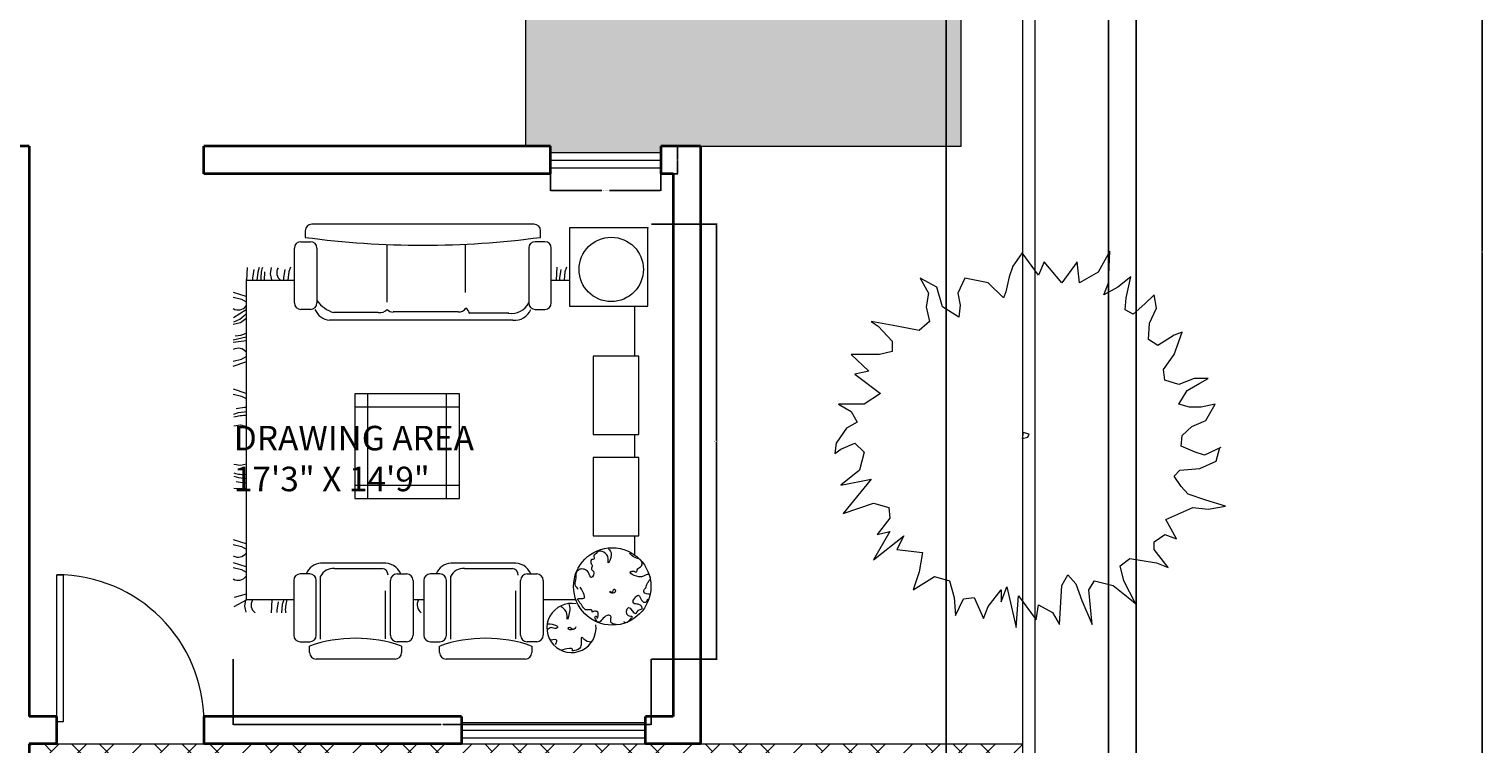
# Model space of a CAD drawing. Units: inches. Extents: x -4843 to -3402, y -164 to 3629.
# Tile 6 of 22: x -4303 to -3829, y 457 to 691. Entities that reach past the tile are written whole.
import ezdxf

# ---------------------------------------------------------------- set-up
doc = ezdxf.new("R2010")
doc.units = ezdxf.units.IN
for name, color, linetype, lineweight in [('A-ANNO-DIMS', 2, 'Continuous', 18), ('A-AREA-IDEN', 2, 'Continuous', 18), ('A-FLOR-DECK', 7, 'Continuous', 18), ('C-PROP', 7, 'Continuous', 25), ('C-PVMT', 7, 'Continuous', 18), ('doors', 2, 'Continuous', 18), ('furniture', 6, 'Continuous', 18), ('L-PLNT-EDGE', 7, 'Continuous', 18), ('PLANTS', 3, 'Continuous', 13), ('walls', 7, 'Continuous', 35), ('windows', 1, 'Continuous', 18)]:
    doc.layers.add(name, color=color, linetype=linetype, lineweight=lineweight)
doc.layers.add('A-FLOR-PATT', color=30, linetype='Continuous', lineweight=13, true_color=0xf26722)
doc.layers.add('C-PVMT-PATT', color=9, linetype='Continuous', lineweight=13, true_color=0xc7c8ca)
doc.styles.get("Standard").update_dxf_attribs({"font": 'arial.ttf'})
doc.dimstyles.get("Standard").update_dxf_attribs({"dimtxt": 0.18, "dimasz": 0.18, "dimexe": 0.18, "dimexo": 0.0625, "dimgap": 0.09, "dimtad": 0, "dimtih": 1, "dimtoh": 1, "dimdec": 4, "dimzin": 0, "dimdsep": 46, "dimtxsty": 'Standard', "dimcen": 0.09, "dimadec": 0, "dimazin": 0, "dimtfac": 1, "dimtdec": 4, "dimtofl": 0, "dimtmove": 0, "dimatfit": 3, "dimfxl": 1, "dimtolj": 1, "dimtzin": 0, "dimarcsym": 0})
pattern_1 = [(45, (-7766.296, -1992.247), (-4.490128, 4.490128), []), (135, (-7766.296, -1992.247), (-13.470384, 4.490128), [15.875, -9.525])]

# ---------------------------------------------------------------- blocks, each defined once
blk = doc.blocks.new('window')
at = {"layer": 'windows'}
for p, q in [((0, 7), (60, 7)), ((0, 4.5), (60, 4.5)), ((0, 2), (60, 2))]:
    blk.add_line(p, q, dxfattribs=at)
for points in [[(0, 9), (0, 0)], [(60, 0), (60, 9)]]:
    blk.add_lwpolyline(points, dxfattribs=at)
blk = doc.blocks.new('windw 3')
at = {"layer": 'windows'}
for p, q in [((0, 7), (36, 7)), ((0, 4.5), (36, 4.5)), ((0, 2), (36, 2))]:
    blk.add_line(p, q, dxfattribs=at)
for points in [[(0, 0), (0, 9)], [(36, 9), (36, 0)]]:
    blk.add_lwpolyline(points, dxfattribs=at)
blk = doc.blocks.new('*U7')
for p, q in [((0, 0), (0, -6)), ((40, 0), (40, -6))]:
    blk.add_line(p, q)
blk.add_lwpolyline([(0, 0), (0, 40), (1.75, 40), (1.75, 0)], close=True)
blk.add_arc((0, 0), 40, 0, 90)
blk = doc.blocks.new('A$C688935E4')
for p, q in [((552, 3277), (552, 3227)), ((2302, 3327), (602, 3327)), ((2352, 3227), (2352, 3277)), ((3173, 3300), (2573, 3300)), ((2573, 3300), (2573, 2700)), ((3173, 2700), (3173, 3300)), ((469, 2725), (469, 3144)), ((519, 3194), (592, 3194)), ((642, 3144), (642, 2725)), ((1175, 3172), (1175, 2731)), ((1775, 3172), (1775, 2805)), ((2261, 3144), (2261, 2725)), ((2384, 3194), (2311, 3194)), ((2434, 2725), (2434, 3144)), ((97, 2899), (469, 2899)), ((102, 454), (102, 2904)), ((108, 2997), (104, 2897)), ((158, 2980), (148, 2916)), ((148, 2916), (148, 2899)), ((189, 2960), (182, 2897)), ((200, 2997), (189, 2960)), ((240, 2963), (237, 2899)), ((291, 2997), (283, 2947)), ((283, 2947), (295, 2901)), ((396, 2982), (387, 2917)), ((387, 2917), (387, 2901)), ((428, 2962), (420, 2899)), ((439, 2999), (428, 2962)), ((2434, 2899), (2573, 2899)), ((2475, 2999), (2472, 2899)), ((2507, 2982), (2497, 2917)), ((2497, 2917), (2497, 2901)), ((2538, 2962), (2531, 2899)), ((2549, 2999), (2538, 2962)), ((0, 2807), (98, 2776)), ((2, 2769), (65, 2754)), ((5, 2613), (101, 2675)), ((65, 2754), (100, 2733)), ((592, 2675), (519, 2675)), ((2311, 2675), (2384, 2675)), ((2573, 2700), (3173, 2700)), ((3071, 2700), (3071, 2319)), ((1, 2564), (57, 2576)), ((7, 2581), (51, 2600)), ((51, 2600), (101, 2642)), ((57, 2576), (99, 2607)), ((2140, 2593), (739, 2593)), ((1110, 2651), (768, 2651)), ((1721, 2656), (1224, 2656)), ((2108, 2646), (1810, 2646)), ((1, 2442), (101, 2465)), ((1, 2424), (103, 2437)), ((0, 2242), (98, 2274)), ((2, 2281), (65, 2296)), ((65, 2296), (100, 2316)), ((3103, 2319), (2753, 2319)), ((2753, 2319), (2753, 1719)), ((3103, 1719), (3103, 2319)), ((0, 2067), (98, 2035)), ((2, 2028), (65, 2013)), ((65, 2013), (100, 1993)), ((1732, 2029), (932, 2029)), ((932, 2029), (932, 1229)), ((1032, 1229), (1032, 2029)), ((1632, 1229), (1632, 2029)), ((1732, 1229), (1732, 2029)), ((23, 1918), (87, 1927)), ((43, 1886), (106, 1894)), ((87, 1927), (104, 1927)), ((1732, 1929), (932, 1929)), ((6, 1875), (43, 1886)), ((6, 1785), (56, 1792)), ((56, 1792), (102, 1781)), ((2753, 1719), (3103, 1719)), ((3071, 1719), (3071, 1543)), ((6, 1492), (56, 1484)), ((56, 1484), (102, 1495)), ((3103, 1543), (2753, 1543)), ((2753, 1543), (2753, 943)), ((3103, 943), (3103, 1543)), ((6, 1401), (43, 1390)), ((23, 1358), (87, 1349)), ((43, 1390), (106, 1382)), ((87, 1349), (104, 1349)), ((6, 1308), (106, 1305)), ((1732, 1329), (932, 1329)), ((932, 1229), (1732, 1229)), ((1632, 1229), (1632, 1229)), ((1732, 1329), (1732, 1329)), ((0, 916), (98, 885)), ((2753, 943), (3103, 943)), ((3071, 943), (3071, 797)), ((2, 877), (65, 862)), ((65, 862), (100, 842)), ((0, 740), (98, 709)), ((2, 701), (65, 686)), ((65, 686), (100, 666)), ((1146, 734), (670, 734)), ((775, 694), (1141, 694)), ((2141, 734), (1665, 734)), ((1770, 694), (2136, 694)), ((464, 602), (464, 183)), ((587, 652), (514, 652)), ((637, 183), (637, 602)), ((670, 152), (670, 634)), ((1204, 183), (1204, 602)), ((1254, 652), (1327, 652)), ((1377, 602), (1377, 183)), ((1459, 602), (1459, 183)), ((1582, 652), (1509, 652)), ((1632, 183), (1632, 602)), ((1665, 152), (1665, 634)), ((2199, 183), (2199, 602)), ((2249, 652), (2322, 652)), ((2372, 602), (2372, 183)), ((9, 402), (102, 454)), ((11, 473), (104, 500)), ((95, 455), (88, 405)), ((464, 454), (102, 454)), ((296, 455), (292, 355)), ((388, 455), (377, 418)), ((1167, 155), (1167, 522)), ((1459, 454), (1377, 454)), ((2162, 155), (2162, 522)), ((2621, 454), (2372, 454)), ((88, 405), (99, 359)), ((346, 438), (336, 374)), ((336, 374), (336, 357)), ((377, 418), (370, 355)), ((514, 133), (587, 133)), ((1327, 133), (1254, 133)), ((1509, 133), (1582, 133)), ((2322, 133), (2249, 133)), ((585, 50), (585, 100)), ((1239, 0), (635, 0)), ((1289, 100), (1289, 50)), ((1580, 50), (1580, 100)), ((2234, 0), (1630, 0)), ((2284, 100), (2284, 50))]:
    blk.add_line(p, q)
for centre, radius in [((2892, 2982), 246), ((2900, 556), 296)]:
    blk.add_circle(centre, radius)
for centre, radius, start, end in [((602, 3277), 50, 90, 180), ((1452, 9941), 6774, 262.3653, 277.6347), ((2302, 3277), 50, 0, 90), ((519, 3144), 50, 90, 180), ((592, 3144), 50, 0, 90), ((2311, 3144), 50, 90, 180), ((2384, 3144), 50, 0, 90), ((469, 2919), 256, 162.3499, 184.9697), ((408, 2957), 73.8, 148.9813, 234.4689), ((40, 2745), 73.8, 238.9813, 324.4689), ((519, 2725), 50, 180, 270), ((592, 2725), 50, 270, 0), ((747, 2722), 129, 201.1539, 266.4257), ((860, 2910), 275, 218.1017, 250.3904), ((1120, 2733), 82.5, 263.0888, 316.219), ((1220, 2706), 50.3, 216.9828, 275.0921), ((1731, 2711), 55.5, 259.6951, 333.4351), ((1716, 2606), 102, 22.8336, 50.9061), ((2129, 2794), 149, 261.7696, 332.5418), ((2153, 2725), 133, 264.3783, 337.7856), ((2311, 2725), 50, 180, 270), ((2384, 2725), 50, 270, 0), ((21, 2635), 161, 268.1865, 300.459), ((40, 2305), 73.8, 35.5311, 121.0187), ((84, 1607), 256, 85.0303, 107.6501), ((84, 1669), 256, 252.3499, 274.9697), ((40, 854), 73.8, 238.9813, 324.4689), ((679, 605), 129, 93.5743, 158.8461), ((765, 589), 105, 84.6221, 154.8677), ((1134, 643), 51.7, 0.1551, 82.6921), ((1159, 602), 133, 22.2144, 95.6217), ((1674, 605), 129, 93.5743, 158.8461), ((1760, 589), 105, 84.6221, 154.8677), ((2129, 643), 51.7, 0.1551, 82.6921), ((2154, 602), 133, 22.2144, 95.6217), ((40, 677), 73.8, 238.9813, 324.4689), ((514, 602), 50, 90, 180), ((587, 602), 50, 0, 90), ((1254, 602), 50, 90, 180), ((1327, 602), 50, 0, 90), ((1509, 602), 50, 90, 180), ((1582, 602), 50, 0, 90), ((2249, 602), 50, 90, 180), ((2322, 602), 50, 0, 90), ((212, 415), 73.8, 148.9813, 234.4689), ((656, 377), 256, 162.3499, 184.9697), ((1482, 415), 73.8, 148.9813, 234.4689), ((2588, 238), 188, 79.0531, 7.4753), ((514, 183), 50, 180, 270), ((937, -899), 1059, 70.6126, 109.3874), ((587, 183), 50, 270, 0), ((1254, 183), 50, 180, 270), ((1327, 183), 50, 270, 0), ((1509, 183), 50, 180, 270), ((1932, -899), 1059, 70.6126, 109.3874), ((1582, 183), 50, 270, 0), ((2249, 183), 50, 180, 270), ((2322, 183), 50, 270, 0), ((635, 50), 50, 180, 270), ((1239, 50), 50, 270, 0), ((1630, 50), 50, 180, 270), ((2234, 50), 50, 270, 0)]:
    blk.add_arc(centre, radius, start, end)
for points, knots in [([(2872, 845), (2883, 832), (2907, 803), (2861, 711), (2881, 801), (2803, 845), (2776, 806), (2751, 796), (2769, 759), (2736, 767), (2735, 745), (2735, 729), (2757, 717), (2729, 687), (2772, 671), (2738, 597), (2722, 670), (2689, 689), (2654, 692), (2636, 677), (2616, 660), (2630, 618), (2602, 571), (2628, 547), (2640, 536)], [0, 0, 0, 0, 51.917432, 115.953134, 148.653762, 243.503618, 260.320221, 285.545105, 312.300159, 330.382893, 349.184414, 364.34271, 376.955185, 410.191929, 431.212679, 481.045637, 526.423186, 566.857378, 599.557953, 620.994965, 633.607388, 678.298148, 729.616372, 774.208118, 774.208118, 774.208118, 774.208118]), ([(3193, 497), (3171, 498), (3139, 498), (3141, 537), (3162, 543), (3158, 564), (3172, 582), (3178, 600), (3200, 616), (3176, 666), (3127, 605), (3003, 663), (3064, 677), (3088, 658), (3091, 699), (3124, 704), (3131, 738), (3113, 769), (3068, 773), (3045, 796), (3032, 809)], [0, 0, 0, 0, 53.592527, 74.613275, 89.477172, 107.559926, 127.501946, 155.547132, 163.955427, 205.361526, 244.007616, 348.394114, 372.361442, 391.162931, 417.7523, 451.647222, 476.161445, 506.768106, 548.174139, 601.102996, 601.102996, 601.102996, 601.102996]), ([(2931, 265), (2913, 268), (2875, 273), (2902, 335), (2834, 339), (2809, 262), (2771, 299), (2764, 331), (2787, 328), (2779, 303), (2799, 340), (2788, 367), (2763, 368), (2743, 356), (2748, 379), (2722, 378), (2690, 370), (2672, 410), (2651, 432), (2622, 472), (2715, 450), (2679, 509), (2655, 551)], [0, 0, 0, 0, 45.280034, 92.937377, 119.85705, 202.50888, 236.142072, 256.951553, 269.208667, 281.099788, 301.041808, 334.936757, 361.691781, 371.092526, 386.250821, 398.507936, 434.181286, 480.617605, 503.835785, 537.072526, 575.832818, 664.519513, 664.519513, 664.519513, 664.519513]), ([(2881, 521), (2889, 512), (2904, 496), (2937, 526), (2907, 537), (2904, 518), (2889, 500), (2884, 512), (2881, 518)], [0, 0, 0, 0, 30.606664, 58.014358, 74.023252, 91.35741, 108.174033, 123.037946, 123.037946, 123.037946, 123.037946]), ([(2985, 289), (2992, 285), (3013, 272), (3030, 301), (3066, 331), (2996, 318), (3019, 448), (3076, 310), (3098, 385), (3133, 380), (3121, 432), (3022, 404), (3112, 529), (3118, 434), (3165, 434), (3170, 452), (3172, 461)], [0, 0, 0, 0, 22.639985, 64.891145, 88.109294, 118.425777, 183.827032, 255.421062, 303.81444, 318.972681, 339.993429, 410.655563, 480.815761, 542.675345, 566.457594, 593.046986, 593.046986, 593.046986, 593.046986]), ([(2569, 423), (2572, 410), (2581, 375), (2552, 269), (2560, 365), (2529, 386), (2509, 399)], [0, 0, 0, 0, 44.986397, 121.416439, 163.141462, 232.795961, 232.795961, 232.795961, 232.795961]), ([(2402, 271), (2418, 270), (2442, 269), (2493, 249), (2462, 227), (2432, 251), (2412, 232), (2402, 224)], [0, 0, 0, 0, 54.24811, 86.403653, 101.26755, 140.368354, 175.036649, 175.036649, 175.036649, 175.036649]), ([(2622, 247), (2617, 239), (2606, 219), (2549, 226), (2578, 251), (2587, 229), (2599, 231), (2604, 232)], [0, 0, 0, 0, 29.429031, 69.090853, 83.95475, 102.989865, 117.853741, 117.853741, 117.853741, 117.853741]), ([(2465, 111), (2472, 124), (2489, 155), (2451, 149), (2429, 146)], [0, 0, 0, 0, 34.795552, 82.452812, 82.452812, 82.452812, 82.452812]), ([(2738, 131), (2718, 133), (2692, 135), (2662, 180), (2660, 126), (2665, 84), (2627, 67), (2592, 61), (2601, 83), (2552, 80), (2529, 73), (2512, 69)], [0, 0, 0, 0, 60.194174, 81.21491, 114.451654, 156.176677, 217.38995, 226.308276, 238.199396, 262.71358, 323.346586, 323.346586, 323.346586, 323.346586])]:
    blk.add_open_spline(points, degree=3, knots=knots)
blk.add_point((3173, 3300))
blk = doc.blocks.new('*U34')
for points in [[(0, 1540.256), (-77.4954, 1428.4452), (-106.5784, 1341.501), (-135.636, 1217.295), (-155.0162, 1167.6126), (-280.9748, 1291.8186), (-474.7514, 1329.0804), (-532.892, 1204.8744), (-513.5118, 1105.5096), (-523.1892, 1006.1194), (-658.8506, 1093.089), (-707.2884, 1254.5568), (-842.9244, 1329.0804), (-775.1064, 1204.8744), (-794.4866, 1093.089), (-765.429, 968.8576), (-852.6272, 894.334), (-1036.701, 931.5958), (-1249.8832, 968.8576), (-1191.7426, 931.5958), (-1075.4614, 807.3898), (-1075.4614, 720.4456), (-1182.0398, 695.6044), (-1414.5768, 695.6044), (-1269.238, 558.9524), (-1385.5192, 534.1112), (-1172.3624, 372.6434), (-1307.9984, 285.6992), (-1521.1552, 285.6992), (-1414.5768, 223.5962), (-1366.139, 136.652), (-1453.3372, 86.9442), (-1540.5354, -37.2618), (-1550.2382, -124.206), (-1501.775, -86.9442), (-1385.5192, -37.2618), (-1307.9984, -111.7854), (-1346.7588, -260.8326), (-1501.775, -385.064), (-1249.8832, -335.3816), (-1482.3948, -621.0554), (-1230.503, -534.1112), (-1104.5444, -571.373), (-1094.8416, -658.3172), (-1201.42, -794.9692), (-1094.8416, -770.128), (-1230.503, -1006.1194), (-978.5858, -807.3898), (-1036.701, -919.1752), (-823.5442, -944.0164), (-852.6272, -1105.4842), (-901.065, -1254.5568), (-726.6686, -1142.746), (-600.71, -1180.0078), (-561.9496, -1316.6598), (-552.2722, -1465.707), (-484.4542, -1329.0804), (-397.2306, -1316.6598), (-319.7352, -1490.5482), (-280.9748, -1391.1834), (-174.3964, -1254.5568), (-174.3964, -1353.9216), (-125.9586, -1229.7156), (-48.4378, -1565.0718), (-29.0576, -1304.2392), (116.2812, -1502.9688), (135.6614, -1378.7628), (251.9172, -1440.8658), (310.0578, -1540.2306), (329.438, -1217.295), (377.8758, -1130.3254), (445.6938, -1204.8744), (494.157, -1341.501), (581.3552, -1540.2306), (552.2722, -1254.5568), (600.71, -1180.0078), (755.7516, -1217.295), (891.3876, -1329.0804), (939.8254, -1366.3422), (842.9498, -1180.0078), (813.8668, -1055.8018), (891.3876, -993.6988), (1114.2472, -1030.9606), (1211.1228, -1068.2224), (1094.867, -919.1752), (1094.867, -857.0722), (1182.0652, -794.9692), (1278.9408, -832.231), (1191.7426, -670.7378), (1414.6022, -571.373), (1540.5608, -583.7936), (1685.8996, -558.9524), (1521.1806, -509.27), (1375.8418, -459.5876), (1317.7012, -397.4846), (1259.5606, -310.515), (1308.0238, -260.8326), (1472.7174, -248.412), (1608.3788, -186.309), (1637.4364, -74.5236)], [(1647.1392, -74.5236), (1511.4778, -136.6266), (1433.9824, -111.7854), (1317.7012, -62.103), (1327.404, 24.8412), (1404.8994, 99.3648), (1521.1806, 149.0726), (1598.676, 285.6992), (1482.4202, 260.858), (1385.5192, 260.858), (1298.321, 285.6992), (1366.139, 397.4846), (1472.7174, 459.5876), (1540.5608, 496.8494), (1424.2796, 496.8494), (1298.321, 447.167), (1182.0652, 484.4288), (1172.3624, 571.3984), (1259.5606, 695.6044), (1327.404, 881.9134), (1259.5606, 857.0722), (1123.9246, 770.128), (1046.4038, 819.8104), (1056.1066, 956.437), (1114.2472, 1080.6684), (1094.867, 1192.4538), (1017.3462, 1117.9302), (920.4452, 1030.9606), (852.6272, 1068.2478), (862.33, 1167.6126), (901.0904, 1341.501), (794.512, 1254.5568), (678.2308, 1192.4538), (716.9912, 1291.8186), (726.6686, 1552.6766), (629.793, 1378.7628), (474.7768, 1291.8186), (455.3966, 1465.7324), (329.438, 1291.8186), (184.0992, 1465.7324), (135.6614, 1353.9216), (0, 1540.256)]]:
    blk.add_lwpolyline(points)
blk.add_lwpolyline([(9.7028, 49.6824), (0, 0), (48.4378, 12.4206), (58.1406, 37.2618)], close=True)
blk = doc.blocks.new('*D38')
at = {"layer": 'A-ANNO-DIMS', "color": 0, "lineweight": -2, "transparency": 16777216}
for p, q in [((-4132.78, 643.29), (-4132.78, 637.77)), ((-4096.78, 643.29), (-4096.78, 637.77)), ((-4132.6, 637.95), (-4116.02, 637.95)), ((-4096.96, 637.95), (-4113.55, 637.95))]:
    blk.add_line(p, q, dxfattribs=at)
at = {"layer": 'A-ANNO-DIMS', "color": 0, "transparency": 16777216}
for points in [[(-4132.6, 637.98), (-4132.6, 637.92), (-4132.78, 637.95)], [(-4096.96, 637.98), (-4096.96, 637.92), (-4096.78, 637.95)]]:
    blk.add_solid(points, dxfattribs=at)
at = {"layer": 'Defpoints', "color": 0, "transparency": 16777216}
for p in [(-4132.78, 643.35), (-4096.78, 643.35), (-4096.78, 637.95)]:
    blk.add_point(p, dxfattribs=at)
at = {"layer": 'A-ANNO-DIMS', "color": 0, "transparency": 16777216, "insert": (-4114.78, 637.95), "char_height": 0.18, "attachment_point": 5}
blk.add_mtext('\\A1;WINDOW B 36 TYP.', dxfattribs=at)
blk = doc.blocks.new('*D39')
at = {"layer": 'A-ANNO-DIMS', "color": 0, "lineweight": -2, "transparency": 16777216}
for p, q in [((-4096.72, 652.35), (-4091.2, 652.35)), ((-4091.38, 652.17), (-4091.38, 648.04)), ((-4091.38, 643.53), (-4091.38, 647.67)), ((-4096.72, 643.35), (-4091.2, 643.35))]:
    blk.add_line(p, q, dxfattribs=at)
at = {"layer": 'A-ANNO-DIMS', "color": 0, "transparency": 16777216}
for points in [[(-4091.41, 652.17), (-4091.35, 652.17), (-4091.38, 652.35)], [(-4091.41, 643.53), (-4091.35, 643.53), (-4091.38, 643.35)]]:
    blk.add_solid(points, dxfattribs=at)
at = {"layer": 'Defpoints', "color": 0, "transparency": 16777216}
for p in [(-4096.78, 652.35), (-4091.38, 652.35), (-4096.78, 643.35)]:
    blk.add_point(p, dxfattribs=at)
at = {"layer": 'A-ANNO-DIMS', "color": 0, "transparency": 16777216, "insert": (-4091.38, 647.85), "char_height": 0.18, "attachment_point": 5}
blk.add_mtext('\\A1;9 TYP.', dxfattribs=at)
blk = doc.blocks.new('*D48')
at = {"layer": 'A-ANNO-DIMS', "color": 0, "lineweight": -2, "transparency": 16777216}
for p, q in [((-4099.85, 626.91), (-4078.45, 626.91)), ((-4078.63, 626.73), (-4078.63, 556.15)), ((-4078.63, 485.2), (-4078.63, 555.78)), ((-4099.85, 485.02), (-4078.45, 485.02))]:
    blk.add_line(p, q, dxfattribs=at)
at = {"layer": 'A-ANNO-DIMS', "color": 0, "transparency": 16777216}
for points in [[(-4078.66, 626.73), (-4078.6, 626.73), (-4078.63, 626.91)], [(-4078.66, 485.2), (-4078.6, 485.2), (-4078.63, 485.02)]]:
    blk.add_solid(points, dxfattribs=at)
at = {"layer": 'Defpoints', "color": 0, "transparency": 16777216}
for p in [(-4099.91, 626.91), (-4078.63, 626.91), (-4099.91, 485.02)]:
    blk.add_point(p, dxfattribs=at)
at = {"layer": 'A-ANNO-DIMS', "color": 0, "transparency": 16777216, "insert": (-4078.63, 555.97), "char_height": 0.18, "attachment_point": 5}
blk.add_mtext('\\A1;LOUNGE SUITE 142', dxfattribs=at)
blk = doc.blocks.new('*D49')
at = {"layer": 'A-ANNO-DIMS', "color": 0, "lineweight": -2, "transparency": 16777216}
for p, q in [((-4236.28, 484.96), (-4236.28, 463.56)), ((-4099.91, 484.96), (-4099.91, 463.56)), ((-4236.1, 463.74), (-4168.38, 463.74)), ((-4100.09, 463.74), (-4167.82, 463.74))]:
    blk.add_line(p, q, dxfattribs=at)
at = {"layer": 'A-ANNO-DIMS', "color": 0, "transparency": 16777216}
for points in [[(-4236.1, 463.77), (-4236.1, 463.71), (-4236.28, 463.74)], [(-4100.09, 463.77), (-4100.09, 463.71), (-4099.91, 463.74)]]:
    blk.add_solid(points, dxfattribs=at)
at = {"layer": 'Defpoints', "color": 0, "transparency": 16777216}
for p in [(-4236.28, 485.02), (-4099.91, 485.02), (-4099.91, 463.74)]:
    blk.add_point(p, dxfattribs=at)
at = {"layer": 'A-ANNO-DIMS', "color": 0, "transparency": 16777216, "insert": (-4168.1, 463.74), "char_height": 0.18, "attachment_point": 5}
blk.add_mtext('\\A1;136', dxfattribs=at)
blk = doc.blocks.new('*D61')
at = {"layer": 'A-ANNO-DIMS', "color": 0, "lineweight": -2, "transparency": 16777216}
for p, q in [((-3941.72, 1149.35), (-3828.78, 1149.35)), ((-3828.96, 1149.17), (-3828.96, 618.04)), ((-3828.96, 86.53), (-3828.96, 617.67)), ((-3941.72, 86.35), (-3828.78, 86.35))]:
    blk.add_line(p, q, dxfattribs=at)
at = {"layer": 'A-ANNO-DIMS', "color": 0, "transparency": 16777216}
for points in [[(-3828.99, 1149.17), (-3828.93, 1149.17), (-3828.96, 1149.35)], [(-3828.99, 86.53), (-3828.93, 86.53), (-3828.96, 86.35)]]:
    blk.add_solid(points, dxfattribs=at)
at = {"layer": 'Defpoints', "color": 0, "transparency": 16777216}
for p in [(-3941.78, 1149.35), (-3828.96, 1149.35), (-3941.78, 86.35)]:
    blk.add_point(p, dxfattribs=at)
at = {"layer": 'A-ANNO-DIMS', "color": 0, "transparency": 16777216, "insert": (-3828.96, 617.85), "char_height": 0.18, "attachment_point": 5}
blk.add_mtext('\\A1;1063', dxfattribs=at)
blk = doc.blocks.new('*D81')
at = {"layer": 'A-ANNO-DIMS', "color": 0, "lineweight": -2, "transparency": 16777216}
for p, q in [((-4332.78, 86.42), (-4332.78, 1392.95)), ((-4332.6, 1392.77), (-4168.61, 1392.77)), ((-4003.86, 1392.77), (-4167.86, 1392.77)), ((-4003.68, 86.42), (-4003.68, 1392.95))]:
    blk.add_line(p, q, dxfattribs=at)
at = {"layer": 'A-ANNO-DIMS', "color": 0, "transparency": 16777216}
for points in [[(-4332.6, 1392.8), (-4332.6, 1392.74), (-4332.78, 1392.77)], [(-4003.86, 1392.8), (-4003.86, 1392.74), (-4003.68, 1392.77)]]:
    blk.add_solid(points, dxfattribs=at)
at = {"layer": 'Defpoints', "color": 0, "transparency": 16777216}
for p in [(-4003.68, 1392.77), (-4332.78, 86.35), (-4003.68, 86.35)]:
    blk.add_point(p, dxfattribs=at)
at = {"layer": 'A-ANNO-DIMS', "color": 0, "transparency": 16777216, "insert": (-4168.23, 1392.77), "char_height": 0.18, "attachment_point": 5}
blk.add_mtext('\\A1;329.1', dxfattribs=at)

msp = doc.modelspace()

# ---------------------------------------------------------------- hatches: boundary and pattern name
at = {"layer": 'A-FLOR-PATT', "transparency": 33554472}
h = msp.add_hatch(color=256, dxfattribs=at)
h.dxf.hatch_style = 1
h.paths.add_polyline_path([(-4538.62, 643.09), (-4595.62, 643.09), (-4666.62, 643.09), (-4666.62, 466.09), (-4595.62, 466.09), (-4538.62, 466.09)])
h.paths.add_polyline_path([(-3998.62, 888.09), (-4083.62, 888.09), (-4140.62, 888.09), (-4140.62, 652.09), (-4132.62, 652.09), (-4132.62, 650.09), (-4096.62, 650.09), (-4096.62, 652.09), (-4083.62, 652.09), (-3998.62, 652.09)])
at = {"layer": 'C-PVMT-PATT'}
h = msp.add_hatch(dxfattribs=at)
h.set_pattern_fill('ANSI38', color=256, scale=2)
h.set_pattern_definition(pattern_1)
h.paths.add_polyline_path([(-4583.98, 275.35), (-4595.78, 275.35), (-4595.78, 324.35), (-4595.78, 373.35), (-4595.78, 466.35), (-4696.78, 466.35), (-4696.78, 95.35), (-4583.98, 95.35), (-4583.98, 226.6)])
h.paths.add_polyline_path([(-4302.78, 226.6), (-4583.98, 226.6), (-4583.98, 95.35), (-4332.78, 95.35), (-4332.78, 86.35), (-4003.68, 86.35), (-4003.68, 95.35), (-3978.78, 95.35), (-3978.78, 457.35), (-4003.68, 457.35), (-4003.68, 139.54), (-4302.78, 139.54)])
h = msp.add_hatch(dxfattribs=at)
h.set_pattern_fill('ANSI38', color=256, scale=2)
h.set_pattern_definition(pattern_1)
h.paths.add_polyline_path([(-4302.78, 139.54), (-4003.68, 139.54), (-4003.68, 457.35), (-4302.78, 457.35)])
edge = h.paths.add_edge_path(flags=16)
edge.add_spline(control_points=[(-4177.52, 219.09), (-4179, 219.51), (-4181.86, 220.31), (-4185.82, 220.95), (-4189.05, 222.54), (-4192.16, 223.72), (-4194.07, 225.9), (-4195.4, 228.28), (-4195.62, 231.06), (-4195.51, 234.52), (-4196.21, 237.87), (-4197.78, 240.97), (-4199.51, 244.96), (-4199.58, 253.67), (-4199.59, 264.61), (-4199.42, 277.52), (-4199.5, 285.22), (-4199.55, 289.24)], knot_values=[0, 0, 0, 0, 0.118823, 0.228347, 0.304709, 0.395218, 0.479661, 0.520666, 0.602694, 0.688012, 0.788383, 0.860898, 0.954729, 1.11959, 1.518327, 1.801929, 2.110556, 2.110556, 2.110556, 2.110556], degree=3, periodic=0)
edge.add_spline(control_points=[(-4199.55, 289.24), (-4200.15, 289.43), (-4201.5, 289.92), (-4203.22, 291.24), (-4204.05, 292.95), (-4204.29, 294.74), (-4202.87, 295.32), (-4201.55, 294.78), (-4200.39, 293.92), (-4199.58, 293.95), (-4199.28, 293.95)], knot_values=[0.088594, 0.088594, 0.088594, 0.088594, 0.13739, 0.198955, 0.245856, 0.290451, 0.306759, 0.353717, 0.391922, 0.414753, 0.414753, 0.414753, 0.414753], degree=3, periodic=0)
edge.add_spline(control_points=[(-4199.28, 293.95), (-4199.27, 294.13), (-4199.06, 299.13), (-4199.65, 310.26), (-4199.6, 321.33), (-4199.56, 327.57), (-4199.56, 327.7)], knot_values=[0.114046, 0.114046, 0.114046, 0.114046, 0.127519, 0.499235, 0.968453, 0.97871, 0.97871, 0.97871, 0.97871], degree=3, periodic=0)
edge.add_spline(control_points=[(-4199.56, 327.7), (-4199.52, 333.71), (-4199.44, 344.59), (-4199.46, 358.57), (-4199.46, 371.83), (-4198.54, 381.94), (-4199.67, 389.9), (-4198.28, 392.53), (-4197.33, 394.06), (-4195.97, 395.69), (-4195, 397.6), (-4194.23, 399.23), (-4194.68, 400.94), (-4193.76, 402.97), (-4192.49, 405.22), (-4190.13, 407.38), (-4184.96, 408.73), (-4176.56, 410.07), (-4163.62, 409.97), (-4150.19, 408.84), (-4138.94, 409.12), (-4131.82, 408.55), (-4128.06, 406.62), (-4125.85, 404.38), (-4124.25, 401.52), (-4124.52, 397.93), (-4122.42, 395.33), (-4121.46, 393.05), (-4120.15, 391.68), (-4119.47, 383.28), (-4119.55, 374.78), (-4119.57, 366.71), (-4119.57, 365.74)], knot_values=[0.97871, 0.97871, 0.97871, 0.97871, 1.440308, 1.814622, 2.054514, 2.455224, 2.610949, 2.635875, 2.681833, 2.750323, 2.797084, 2.847368, 2.883024, 2.926275, 3.011124, 3.084414, 3.16311, 3.41524, 3.739789, 4.152943, 4.449449, 4.607544, 4.693588, 4.767288, 4.84799, 4.936972, 5.028501, 5.093159, 5.12765, 5.168553, 5.718196, 5.794044, 5.794044, 5.794044, 5.794044], degree=3, periodic=0)
edge.add_spline(control_points=[(-4120.18, 367.25), (-4120.14, 367.18), (-4119.97, 366.93), (-4119.55, 366.17), (-4119.49, 364.82), (-4119.6, 363.39), (-4120.03, 362.65), (-4120.18, 362.38)], knot_values=[0, 0, 0, 0, 0.00069, 0.002823, 0.007863, 0.012889, 0.015703, 0.015703, 0.015703, 0.015703], degree=3, periodic=0)
edge.add_spline(control_points=[(-4119.57, 364.08), (-4119.56, 351.01), (-4119.42, 337.76), (-4119.41, 324.56)], knot_values=[5.836848, 5.836848, 5.836848, 5.836848, 6.848265, 6.848265, 6.848265, 6.848265], degree=3, periodic=0)
edge.add_ellipse((-4119.53, 321.37), major_axis=(-0.07, 3.66), ratio=0.102782, start_angle=-179.3184, end_angle=-3.3021, ccw=False)
edge.add_spline(control_points=[(-4119.41, 317.74), (-4119.43, 309.85), (-4119.49, 301.98), (-4119.55, 294.11)], knot_values=[7.022686, 7.022686, 7.022686, 7.022686, 7.62832, 7.62832, 7.62832, 7.62832], degree=3, periodic=0)
edge.add_spline(control_points=[(-4119.55, 294.11), (-4119.55, 294.04), (-4119.54, 293.98), (-4119.53, 293.92)], knot_values=[3.166598, 3.166598, 3.166598, 3.166598, 3.17144, 3.17144, 3.17144, 3.17144], degree=3, periodic=0)
edge.add_spline(control_points=[(-4119.53, 293.92), (-4119.49, 293.93), (-4118.98, 293.99), (-4117.92, 293.82), (-4116.62, 294.78), (-4115.3, 295.32), (-4113.88, 294.74), (-4114.12, 292.95), (-4114.96, 291.24), (-4116.83, 289.8), (-4118.38, 289.3), (-4119.18, 289.17)], knot_values=[0.073944, 0.073944, 0.073944, 0.073944, 0.077675, 0.113045, 0.15125, 0.198208, 0.214516, 0.259111, 0.306012, 0.367577, 0.431023, 0.431023, 0.431023, 0.431023], degree=3, periodic=0)
edge.add_spline(control_points=[(-4119.18, 289.17), (-4119.16, 288.25), (-4119.23, 285.31), (-4120.26, 281.21), (-4116.4, 269.66), (-4119.27, 257.62), (-4120.12, 246.29), (-4120, 242.31), (-4122.07, 238.8), (-4123.28, 234.04), (-4123.32, 229.29), (-4124.68, 225.36), (-4128.1, 222.41), (-4132.86, 220.91), (-4139.06, 219.63), (-4143.16, 218.66), (-4145.64, 218.22)], knot_values=[0.819302, 0.819302, 0.819302, 0.819302, 0.890194, 1.044711, 1.132212, 1.809474, 1.943489, 2.01252, 2.108859, 2.247504, 2.386276, 2.473581, 2.556705, 2.722147, 2.850835, 3.044752, 3.044752, 3.044752, 3.044752], degree=3, periodic=0)
edge.add_spline(control_points=[(-4145.64, 218.22), (-4146.33, 218.09), (-4151.86, 217.2), (-4162, 217.3), (-4171.27, 218.35), (-4175.68, 218.87)], knot_values=[0.047426, 0.047426, 0.047426, 0.047426, 0.101273, 0.477921, 0.819302, 0.819302, 0.819302, 0.819302], degree=3, periodic=0)
edge.add_spline(control_points=[(-4175.68, 218.87), (-4176.29, 218.95), (-4176.91, 219.02), (-4177.52, 219.09)], knot_values=[0, 0, 0, 0, 0.047426, 0.047426, 0.047426, 0.047426], degree=3, periodic=0)
edge = h.paths.add_edge_path(flags=0)
edge.add_spline(control_points=[(-4193.77, 273.03), (-4191.09, 287.2), (-4187.62, 302.4), (-4186.93, 321.11), (-4186.81, 324.35), (-4186.61, 327.58)], knot_values=[0.011622, 0.011622, 0.011622, 0.011622, 0.154395, 0.154395, 0.1842, 0.1842, 0.1842, 0.1842], degree=3, periodic=0)
edge.add_arc((-14109, 562.63), 9925.18, 358.64295, 358.862544)
edge.add_arc((-4243.78, 366.9), 58.02, 358.7216, 381.1082)
edge.add_arc((-4190.02, 387.65), 0.39, 21.1082, 164.1707)
edge.add_arc((-4151.78, 376.81), 40.14, 164.1707, 171.876)
edge.add_spline(control_points=[(-4191.52, 382.48), (-4193.63, 363.98), (-4194.06, 359.93), (-4194.6, 348.28), (-4195.39, 329.61), (-4195.57, 309.17), (-4194.94, 291.19), (-4195.23, 280.27), (-4195.7, 273.24)], knot_values=[0.04998, 0.04998, 0.04998, 0.04998, 0.066649, 0.35819, 0.953971, 1.497659, 1.929861, 2.336539, 2.336539, 2.336539, 2.336539], degree=3, periodic=0)
edge.add_arc((-4194.73, 273.21), 0.976, 178.3008, 349.1958)
edge = h.paths.add_edge_path(flags=0)
edge.add_spline(control_points=[(-4195.31, 273.22), (-4195.21, 274.79), (-4195.12, 276.28), (-4195.04, 277.7)], knot_values=[0.050139, 0.050139, 0.050139, 0.050139, 0.140986, 0.140986, 0.140986, 0.140986], degree=3, periodic=0)
edge.add_line((-4195.04, 277.7), (-4193.1, 278.54))
edge.add_spline(control_points=[(-4193.1, 278.54), (-4193.46, 276.71), (-4193.81, 274.9), (-4194.15, 273.1)], knot_values=[0.011622, 0.011622, 0.011622, 0.011622, 0.029731, 0.029731, 0.029731, 0.029731], degree=3, periodic=0)
edge.add_arc((-4194.73, 273.21), 0.586, 178.9277, 349.1656, ccw=False)
edge = h.paths.add_edge_path(flags=0)
edge.add_spline(control_points=[(-4192.94, 267.88), (-4190.53, 282.97), (-4186.3, 296.57), (-4184.85, 314.75), (-4184.63, 317.86), (-4184.63, 317.86)], knot_values=[0.000364, 0.000364, 0.000364, 0.000364, 0.134701, 0.134701, 0.150836, 0.150836, 0.150836, 0.150836], degree=3, periodic=0)
edge.add_spline(control_points=[(-4184.63, 317.86), (-4184.48, 319.61), (-4184.14, 329.7), (-4184.58, 344.88), (-4184.71, 357.85), (-4185.28, 371.27)], knot_values=[0.036478, 0.036478, 0.036478, 0.036478, 0.053439, 0.129277, 0.173634, 0.173634, 0.173634, 0.173634], degree=3, periodic=0)
edge.add_arc((-4181.38, 371.43), 3.9, 95.3633, 182.3534, ccw=False)
edge.add_spline(control_points=[(-4181.75, 375.32), (-4178.43, 375.63), (-4172.02, 376.65), (-4161.57, 377.87), (-4149.14, 377.13), (-4140.59, 376.64), (-4136.44, 375.2)], knot_values=[0.007384, 0.007384, 0.007384, 0.007384, 0.029401, 0.067193, 0.103796, 0.144479, 0.144479, 0.144479, 0.144479], degree=3, periodic=0)
edge.add_arc((-4137.72, 371.51), 3.9, -1.298, 70.8366, ccw=False)
edge.add_spline(control_points=[(-4133.81, 371.42), (-4133.92, 366.8), (-4133.8, 365.25), (-4134.1, 356.56), (-4133.51, 346.62), (-4132.74, 328.68), (-4132.62, 320.9), (-4131.51, 309.76), (-4131.36, 307.85), (-4131.08, 305.65)], knot_values=[0.107006, 0.107006, 0.107006, 0.107006, 0.118332, 0.118332, 0.206466, 0.206466, 0.276418, 0.276418, 0.309317, 0.309317, 0.309317, 0.309317], degree=3, periodic=0)
edge.add_arc((-3971.07, 314.1), 160.23, 183.0239, 196.3405)
edge.add_arc((-4128.58, 267.92), 3.9, -60.024, 16.3405, ccw=False)
edge.add_arc((-4159.42, 321.39), 65.63, 241.2771, 299.976, ccw=False)
edge.add_arc((-4189.08, 267.26), 3.9, 170.9279, 241.2771, ccw=False)
edge = h.paths.add_edge_path(flags=0)
edge.add_spline(control_points=[(-4194.99, 278.72), (-4194.87, 281.24), (-4194.79, 283.56), (-4194.71, 288.07), (-4194.71, 290.31), (-4194.73, 292.52)], knot_values=[0.163087, 0.163087, 0.163087, 0.163087, 0.328206, 0.328206, 0.498586, 0.498586, 0.498586, 0.498586], degree=3, periodic=0)
edge.add_line((-4194.73, 292.52), (-4189.99, 295.11))
edge.add_spline(control_points=[(-4189.99, 295.11), (-4190.88, 289.87), (-4191.9, 284.7), (-4192.89, 279.64)], knot_values=[0.033336, 0.033336, 0.033336, 0.033336, 0.083278, 0.083278, 0.083278, 0.083278], degree=3, periodic=0)
edge.add_line((-4192.89, 279.64), (-4194.99, 278.72))
edge = h.paths.add_edge_path(flags=0)
edge.add_spline(control_points=[(-4178.7, 221.84), (-4179.39, 222.03), (-4180.88, 222.44), (-4183.38, 222.93), (-4185.9, 223.59), (-4189.06, 224.07), (-4191.51, 226.12), (-4193.19, 228.61), (-4194.59, 231.18), (-4194.2, 234.35), (-4194.53, 237.78), (-4194.39, 240.52), (-4195.15, 242.77), (-4194.42, 243.88), (-4193.69, 245.31), (-4192.7, 244.3), (-4192.76, 242.61), (-4192.13, 240.02), (-4191.54, 236.65), (-4189.84, 233.5), (-4187.61, 230.62), (-4184.55, 228.88), (-4182.1, 227.6), (-4180.18, 227.57), (-4179.35, 226.59), (-4178.67, 225.18), (-4178.52, 223.73), (-4177.56, 222.16), (-4178.35, 221.94), (-4178.7, 221.84)], knot_values=[0, 0, 0, 0, 0.048183, 0.105687, 0.173148, 0.226645, 0.320656, 0.377708, 0.433539, 0.514499, 0.587235, 0.668333, 0.704408, 0.73448, 0.764541, 0.77911, 0.812729, 0.87811, 0.959931, 1.044551, 1.119493, 1.20463, 1.28096, 1.307559, 1.326943, 1.363733, 1.411478, 1.437083, 1.45761, 1.45761, 1.45761, 1.45761], degree=3, periodic=0)
edge = h.paths.add_edge_path(flags=0)
edge.add_spline(control_points=[(-4188.52, 267.77), (-4189.01, 267.9), (-4189.74, 268.12), (-4190.47, 268.86), (-4190.7, 270.15), (-4190.08, 273.88), (-4189.7, 277.37), (-4189.34, 280.09)], knot_values=[0, 0, 0, 0, 0.038062, 0.057765, 0.075887, 0.136118, 0.346676, 0.346676, 0.346676, 0.346676], degree=3, periodic=0)
edge.add_spline(control_points=[(-4189.34, 280.09), (-4189.32, 280.27), (-4188.86, 283.67), (-4188.3, 287.07), (-4187.7, 290.25)], knot_values=[0.346676, 0.346676, 0.346676, 0.346676, 0.360736, 0.61029, 0.61029, 0.61029, 0.61029], degree=3, periodic=0)
edge.add_spline(control_points=[(-4187.7, 290.25), (-4187.64, 290.55), (-4187.59, 290.84), (-4187.53, 291.13)], knot_values=[0.61029, 0.61029, 0.61029, 0.61029, 0.63318, 0.63318, 0.63318, 0.63318], degree=3, periodic=0)
edge.add_spline(control_points=[(-4187.53, 291.13), (-4187.46, 291.48), (-4186.97, 294.04), (-4186.21, 297.64), (-4185.68, 301.41), (-4185.64, 302.9), (-4185.53, 303.78), (-4182.16, 302.88), (-4174.34, 302.04), (-4164.13, 301.75), (-4156.84, 301.61), (-4156.19, 301.6)], knot_values=[0.63318, 0.63318, 0.63318, 0.63318, 0.660851, 0.833831, 0.919425, 0.944413, 0.95681, 0.976133, 1.15453, 1.659168, 1.709179, 1.709179, 1.709179, 1.709179], degree=3, periodic=0)
edge.add_spline(control_points=[(-4156.19, 301.6), (-4155.1, 301.58), (-4154.03, 301.57), (-4152.95, 301.57)], knot_values=[1.709179, 1.709179, 1.709179, 1.709179, 1.79199, 1.79199, 1.79199, 1.79199], degree=3, periodic=0)
edge.add_spline(control_points=[(-4152.95, 301.57), (-4152.42, 301.57), (-4151.9, 301.57), (-4151.37, 301.57)], knot_values=[1.79199, 1.79199, 1.79199, 1.79199, 1.832683, 1.832683, 1.832683, 1.832683], degree=3, periodic=0)
edge.add_spline(control_points=[(-4151.37, 301.57), (-4150.4, 301.58), (-4145.3, 301.69), (-4139.09, 302.34), (-4133.97, 303.31), (-4132.93, 303.51)], knot_values=[1.832683, 1.832683, 1.832683, 1.832683, 1.908025, 2.226872, 2.308645, 2.308645, 2.308645, 2.308645], degree=3, periodic=0)
edge.add_arc((-4132.85, 303.13), 0.39, 4.7136, 100.9875, ccw=False)
edge.add_arc((-3928.85, 319.95), 204.3, 184.7136, 194.294)
edge.add_arc((-4127.21, 269.41), 0.39, -17.7257, 14.294, ccw=False)
edge.add_spline(control_points=[(-4126.84, 269.29), (-4126.85, 269.25), (-4126.95, 268.96), (-4127.33, 268.39), (-4128.31, 268.05), (-4128.95, 267.71), (-4129.3, 267.52)], knot_values=[0, 0, 0, 0, 0.003035, 0.023811, 0.049681, 0.080112, 0.080112, 0.080112, 0.080112], degree=3, periodic=0)
edge.add_spline(control_points=[(-4129.3, 267.52), (-4133.15, 266.24), (-4140.45, 263.81), (-4151.73, 262.21), (-4163.24, 261.98), (-4173.69, 262.83), (-4182.22, 265.35), (-4186.54, 267.01), (-4188.52, 267.77)], knot_values=[0, 0, 0, 0, 0.276247, 0.522812, 0.772814, 1.060937, 1.232089, 1.37667, 1.37667, 1.37667, 1.37667], degree=3, periodic=0)
edge = h.paths.add_edge_path(flags=0)
edge.add_spline(control_points=[(-4194.74, 293.44), (-4194.76, 295.48), (-4194.8, 297.5), (-4194.95, 304.1), (-4195.06, 308.66), (-4195.08, 316.65), (-4195.06, 320.09), (-4195, 323.53)], knot_values=[0.522233, 0.522233, 0.522233, 0.522233, 0.678921, 0.678921, 1.029636, 1.029636, 1.294056, 1.294056, 1.294056, 1.294056], degree=3, periodic=0)
edge.add_arc((-4194.61, 323.53), 0.39, 118.6584, 180.1243, ccw=False)
edge.add_line((-4194.8, 323.87), (-4187.58, 327.81))
edge.add_arc((-4187.4, 327.47), 0.39, -1.7955, 118.6584, ccw=False)
edge.add_spline(control_points=[(-4187.01, 327.45), (-4187.19, 324.61), (-4187.3, 321.78), (-4187.57, 314.47), (-4187.91, 310.04), (-4188.83, 302.44), (-4189.3, 299.28), (-4189.82, 296.13)], knot_values=[0.086512, 0.086512, 0.086512, 0.086512, 0.1126, 0.1126, 0.153879, 0.153879, 0.183727, 0.183727, 0.183727, 0.183727], degree=3, periodic=0)
edge.add_line((-4189.82, 296.13), (-4194.74, 293.44))
h.paths.add_polyline_path([(-4186.78, 287.12, -0.033695), (-4130.99, 288.38, -0.199929), (-4148.63, 273.2), (-4148.83, 271.67, -0.261093), (-4149.06, 271.36, -0.216615), (-4169.29, 271.5, -0.246093), (-4169.52, 271.79), (-4169.81, 273.49, -0.273701)], flags=0)
edge = h.paths.add_edge_path(flags=0)
edge.add_arc((-4140.72, 295.8), 3.69, -59.0277, 20.0091, ccw=False)
edge.add_arc((-4142.47, 285.34), 8.16, 63.4848, 115.5347)
edge.add_arc((-4143.91, 295.28), 3.32, 152.2145, 231.1029, ccw=False)
edge.add_ellipse((-4142.44, 301.89), major_axis=(10.53, 0), ratio=0.529672, start_angle=218.5261, end_angle=229.0127, ccw=False)
edge.add_spline(control_points=[(-4148.27, 297.25), (-4148.49, 296.95), (-4148.81, 296.44), (-4148.95, 295.85), (-4148.97, 295.61)], knot_values=[0.565799, 0.565799, 0.565799, 0.565799, 0.593545, 0.612564, 0.612564, 0.612564, 0.612564], degree=3, periodic=0)
edge.add_spline(control_points=[(-4148.97, 295.61), (-4149.06, 294.82), (-4148.63, 292.94), (-4147.27, 290.81), (-4145.07, 289.2), (-4142.36, 289.18), (-4139.75, 289.34), (-4137.6, 290.68), (-4136.36, 292.26), (-4136.35, 293.38), (-4136.37, 293.76)], knot_values=[0.086242, 0.086242, 0.086242, 0.086242, 0.147544, 0.220255, 0.282478, 0.345524, 0.423154, 0.480194, 0.536785, 0.565799, 0.565799, 0.565799, 0.565799], degree=3, periodic=0)
edge.add_spline(control_points=[(-4136.37, 293.76), (-4136.39, 293.98), (-4136.52, 295.13), (-4136.68, 296.22), (-4136.81, 297.11)], knot_values=[0, 0, 0, 0, 0.016519, 0.086242, 0.086242, 0.086242, 0.086242], degree=3, periodic=0)
edge.add_ellipse((-4142.44, 301.89), major_axis=(10.53, 0), ratio=0.529672, start_angle=229.0127, end_angle=352.38, ccw=False)
edge = h.paths.add_edge_path(flags=0)
edge.add_ellipse((-4159.28, 300.8), major_axis=(0, 3.41), ratio=0.932272, start_angle=137.9206, end_angle=219.4265)
edge.add_line((-4157.17, 298.24), (-4157.17, 295.16))
edge.add_line((-4157.17, 295.16), (-4152.61, 295.16))
edge.add_arc((-4152.61, 294.77), 0.39, 0, 90, ccw=False)
edge.add_line((-4152.22, 294.77), (-4152.22, 289.6))
edge.add_arc((-4152.61, 289.6), 0.39, -90, 0, ccw=False)
edge.add_line((-4152.61, 289.21), (-4165.23, 289.21))
edge.add_arc((-4165.23, 289.6), 0.39, 180, 270, ccw=False)
edge.add_line((-4165.62, 289.6), (-4165.62, 294.77))
edge.add_arc((-4165.23, 294.77), 0.39, 90, 180, ccw=False)
edge.add_line((-4165.23, 295.16), (-4161.49, 295.16))
edge.add_line((-4161.49, 295.16), (-4161.49, 298.35))
edge = h.paths.add_edge_path(flags=0)
edge.add_ellipse((-4198.94, 321.56), major_axis=(0.07, 3.66), ratio=0.102782, start_angle=0, end_angle=360)

# ---------------------------------------------------------------- linework, layer by layer
at = {"layer": 'A-FLOR-DECK'}
for p, q in [((-4140.78, 652.35), (-4140.78, 888.35)), ((-3998.78, 652.35), (-3998.78, 888.35)), ((-4083.78, 652.35), (-3998.78, 652.35))]:
    msp.add_line(p, q, dxfattribs=at)
at = {"layer": 'C-PROP'}
for p, q in [((-3941.78, 1149.35), (-3941.78, 86.35)), ((-3950.78, 1140.35), (-3950.78, 95.35))]:
    msp.add_line(p, q, dxfattribs=at)
at = {"layer": 'C-PVMT'}
msp.add_line((-4003.68, 457.35), (-3978.78, 457.35), dxfattribs=at)
msp.add_lwpolyline([(-4302.78, 457.35), (-4003.68, 457.35), (-4003.68, 139.54), (-4302.78, 139.54)], close=True, dxfattribs=at)
at = {"layer": 'furniture'}
msp.add_open_spline([(-4113.94, 516.52), (-4113.94, 516.52), (-4113.94, 516.53), (-4113.94, 516.54)], degree=3, dxfattribs=at)
at = {"layer": 'L-PLNT-EDGE'}
for p, q in [((-3974.78, 1116.35), (-3974.78, 95.35)), ((-3978.78, 1112.35), (-3978.78, 95.35))]:
    msp.add_line(p, q, dxfattribs=at)
at = {"layer": 'walls'}
for p, q in [((-4302.78, 652.35), (-4311.78, 652.35)), ((-4302.78, 652.35), (-4302.78, 466.35)), ((-4132.78, 652.35), (-4245.78, 652.35)), ((-4245.78, 643.35), (-4245.78, 652.35)), ((-4083.78, 652.35), (-4096.78, 652.35)), ((-4083.78, 652.35), (-4083.78, 457.35)), ((-4132.78, 643.35), (-4245.78, 643.35)), ((-4092.78, 643.35), (-4096.78, 643.35)), ((-4092.78, 643.35), (-4092.78, 466.35)), ((-4293.78, 466.35), (-4302.78, 466.35)), ((-4161.78, 466.35), (-4245.78, 466.35)), ((-4092.78, 466.35), (-4101.78, 466.35)), ((-4302.78, 457.35), (-4302.78, 275.35)), ((-4293.78, 457.35), (-4302.78, 457.35)), ((-4161.78, 457.35), (-4245.78, 457.35)), ((-4083.78, 457.35), (-4101.78, 457.35))]:
    msp.add_line(p, q, dxfattribs=at)
for points in [[(-4132.78, 643.35), (-4132.78, 652.35)], [(-4096.78, 652.35), (-4096.78, 643.35)], [(-4293.78, 457.35), (-4293.78, 466.35)], [(-4245.78, 466.35), (-4245.78, 457.35)], [(-4161.78, 466.35), (-4161.78, 457.35)], [(-4101.78, 457.35), (-4101.78, 466.35)]]:
    msp.add_lwpolyline(points, dxfattribs=at)

# ---------------------------------------------------------------- block references
at = {"layer": 'doors', "xscale": 1.199999999999999, "yscale": 1.199999999999999, "zscale": 1.199999999999999}
msp.add_blockref('*U7', (-4293.78, 464.55), dxfattribs=at)
at = {"layer": 'furniture', "xscale": 0.0426469850978482, "yscale": 0.0426469850978482, "zscale": 0.0426469850978482}
msp.add_blockref('A$C688935E4', (-4236.28, 485.02), dxfattribs=at)
at = {"layer": 'PLANTS', "xscale": 0.0393700787401575, "yscale": 0.0393700787401575, "zscale": 0.0393700787401575}
msp.add_blockref('*U34', (-3978.97, 556.99), dxfattribs=at)
at = {"layer": 'windows'}
for name, p in [('windw 3', (-4132.78, 643.35)), ('window', (-4161.78, 457.35))]:
    msp.add_blockref(name, p, dxfattribs=at)

# ---------------------------------------------------------------- texts
at = {"layer": 'A-AREA-IDEN', "insert": (-4236.03, 561.14), "char_height": 8, "attachment_point": 1}
msp.add_mtext_dynamic_manual_height_columns('DRAWING AREA \\P17\'3" X 14\'9"', width=97.7596, gutter_width=60, heights=[0], dxfattribs=at)

# ---------------------------------------------------------------- dimensions: what is measured, and where the dimension line sits
at = {"layer": 'A-ANNO-DIMS'}
for base, p1, p2, override, picture, middle in [((-4003.68, 1392.77), (-4332.78, 86.35), (-4003.68, 86.35), {"dimdec": 1, "dimlfac": 1, "dimrnd": 0, "dimzin": 0, "dimdsep": 46, "dimlunit": 2}, '*D81', (-4168.23, 1392.77)), ((-4099.91, 463.74), (-4236.28, 485.02), (-4099.91, 485.02), {"dimdec": 0, "dimlfac": 1, "dimrnd": 0, "dimzin": 0, "dimdsep": 46, "dimlunit": 2}, '*D49', (-4168.1, 463.74))]:
    dim = msp.add_linear_dim(base=base, p1=p1, p2=p2, dimstyle='Standard', override=override, dxfattribs=at)
    dim.commit()
    dim.dimension.update_dxf_attribs({"geometry": picture, "text_midpoint": middle})
dim = msp.add_linear_dim(base=(-3828.96, 1149.35), p1=(-3941.78, 86.35), p2=(-3941.78, 1149.35), angle=90, dimstyle='Standard', override={"dimdec": 0, "dimlfac": 1, "dimrnd": 0, "dimzin": 0, "dimdsep": 46, "dimlunit": 2}, dxfattribs=at)
dim.commit()
dim.dimension.update_dxf_attribs({"geometry": '*D61', "text_midpoint": (-3828.96, 617.85)})
for base, p1, p2, text, picture, middle in [((-4091.38, 652.35), (-4096.78, 643.35), (-4096.78, 652.35), '<> TYP.', '*D39', (-4091.38, 647.85)), ((-4078.63, 626.91), (-4099.91, 485.02), (-4099.91, 626.91), 'LOUNGE SUITE <>', '*D48', (-4078.63, 555.97))]:
    dim = msp.add_linear_dim(base=base, p1=p1, p2=p2, angle=90, text=text, dimstyle='Standard', override={"dimdec": 0, "dimlfac": 1, "dimrnd": 0, "dimzin": 0, "dimdsep": 46, "dimlunit": 2}, dxfattribs=at)
    dim.commit()
    dim.dimension.update_dxf_attribs({"geometry": picture, "text_midpoint": middle})
dim = msp.add_linear_dim(base=(-4096.78, 637.95), p1=(-4132.78, 643.35), p2=(-4096.78, 643.35), text='WINDOW B <> TYP.', dimstyle='Standard', override={"dimdec": 0, "dimlfac": 1, "dimrnd": 0, "dimzin": 0, "dimdsep": 46, "dimlunit": 2}, dxfattribs=at)
dim.commit()
dim.dimension.update_dxf_attribs({"geometry": '*D38', "text_midpoint": (-4114.78, 637.95)})

doc.saveas('drawing.dxf')
